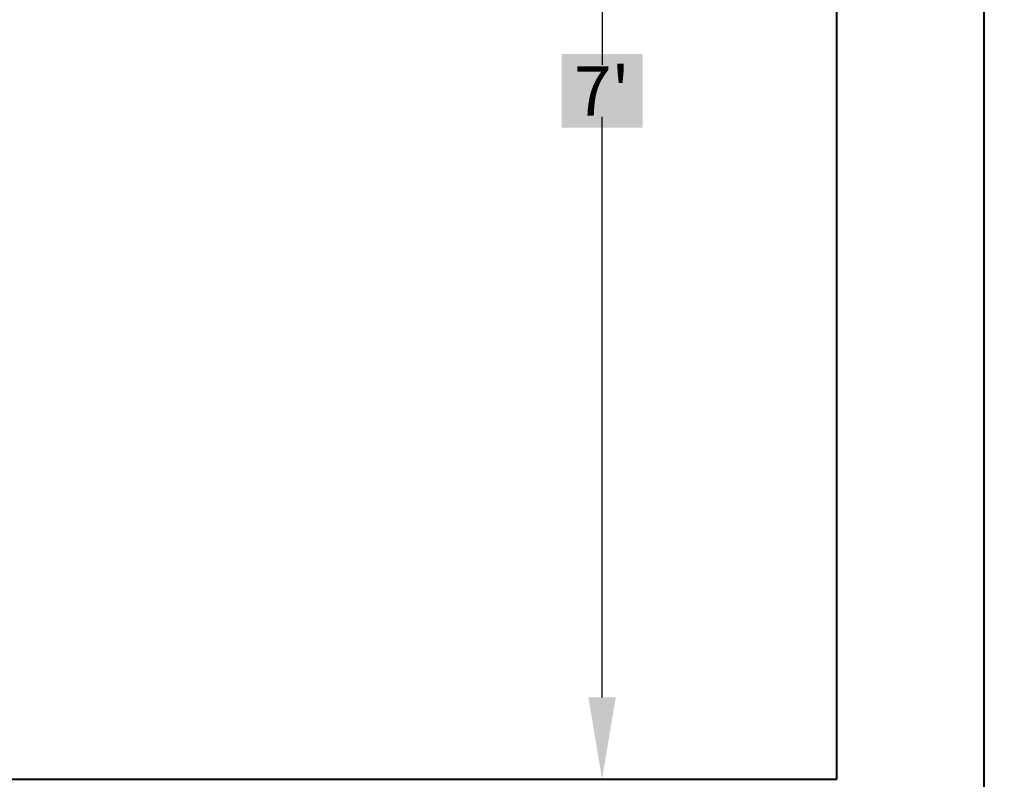
# Model space of a CAD drawing. Units: inches. Extents: x -301 to 715, y -607 to 364.
# Tile 91 of 141: x 74 to 134, y -215 to -168. Entities that reach past the tile are written whole.
import ezdxf

# ---------------------------------------------------------------- set-up
doc = ezdxf.new("R2010")
doc.units = ezdxf.units.IN
doc.header["$MEASUREMENT"] = 0
doc.layers.add('A-ANNO-DIMS', color=2, linetype='Continuous', lineweight=18)
doc.layers.add('A-WALL', color=3, linetype='Continuous', lineweight=40)
doc.styles.get("Standard").update_dxf_attribs({"font": 'arial.ttf'})
doc.dimstyles.get("Standard").update_dxf_attribs({"dimtxt": 0.18, "dimasz": 0.18, "dimexe": 0.18, "dimexo": 0.0625, "dimgap": 0.09, "dimtad": 0, "dimtih": 1, "dimtoh": 1, "dimdec": 1, "dimzin": 0, "dimdsep": 46, "dimlunit": 4, "dimtxsty": 'Standard', "dimcen": 0.09, "dimclrd": 3, "dimclre": 4, "dimclrt": 6, "dimadec": 0, "dimazin": 0, "dimtfac": 1, "dimtdec": 1, "dimtofl": 0, "dimtmove": 0, "dimatfit": 3, "dimfxl": 1, "dimtfill": 2, "dimtfillclr": 51, "dimtolj": 1, "dimtzin": 0, "dimarcsym": 0})

# ---------------------------------------------------------------- blocks, each defined once
blk = doc.blocks.new('*D43')
at = {"layer": 'A-ANNO-DIMS', "color": 0, "lineweight": -2, "transparency": 16777216}
for p, q in [((123.834, -130.818), (109.393, -130.818)), ((109.573, -135.818), (109.573, -171.228)), ((109.573, -209.818), (109.573, -174.408)), ((123.834, -214.818), (109.393, -214.818))]:
    blk.add_line(p, q, dxfattribs=at)
at = {"layer": 'A-ANNO-DIMS', "color": 0, "transparency": 16777216}
for points in [[(108.739, -135.818), (110.406, -135.818), (109.573, -130.818)], [(108.739, -209.818), (110.406, -209.818), (109.573, -214.818)]]:
    blk.add_solid(points, dxfattribs=at)
at = {"layer": 'Defpoints', "color": 0, "transparency": 16777216}
for p in [(123.897, -130.818), (109.573, -214.818), (123.897, -214.818)]:
    blk.add_point(p, dxfattribs=at)
at = {"layer": 'A-ANNO-DIMS', "color": 0, "transparency": 16777216, "insert": (109.573, -172.818), "char_height": 3, "attachment_point": 5, "bg_fill": 1, "box_fill_scale": 1.25, "bg_fill_color": 51, "bg_fill_transparency": 0}
blk.add_mtext("\\A1;7'", dxfattribs=at)
blk = doc.blocks.new('*D152')
at = {"layer": 'A-ANNO-DIMS', "color": 4, "lineweight": -2, "transparency": 16777216}
for p, q in [((123.959, -130.818), (233.659, -130.818)), ((132.959, -223.818), (233.659, -223.818))]:
    blk.add_line(p, q, dxfattribs=at)
at = {"layer": 'A-ANNO-DIMS', "color": 3, "lineweight": -2, "transparency": 16777216}
for p, q in [((233.479, -130.998), (233.479, -177.136)), ((233.479, -223.638), (233.479, -177.5))]:
    blk.add_line(p, q, dxfattribs=at)
at = {"layer": 'A-ANNO-DIMS', "color": 3, "transparency": 16777216}
for points in [[(233.449, -130.998), (233.509, -130.998), (233.479, -130.818)], [(233.449, -223.638), (233.509, -223.638), (233.479, -223.818)]]:
    blk.add_solid(points, dxfattribs=at)
at = {"layer": 'Defpoints', "color": 0, "transparency": 16777216}
for p in [(123.897, -130.818), (233.479, -130.818), (132.897, -223.818)]:
    blk.add_point(p, dxfattribs=at)
at = {"layer": 'A-ANNO-DIMS', "color": 6, "transparency": 16777216, "insert": (233.479, -177.318), "char_height": 0.18, "attachment_point": 5, "bg_fill": 1, "box_fill_scale": 1.25, "bg_fill_color": 51, "bg_fill_transparency": 0}
blk.add_mtext('\\A1;7\'-9"', dxfattribs=at)

msp = doc.modelspace()

# ---------------------------------------------------------------- linework, layer by layer
at = {"layer": 'A-WALL'}
for p, q in [((123.897, -214.818), (123.897, -82.818)), ((132.897, -223.818), (132.897, -124.818)), ((-45.841, -214.818), (123.897, -214.818)), ((123.897, -214.818), (123.897, -214.818))]:
    msp.add_line(p, q, dxfattribs=at)

# ---------------------------------------------------------------- dimensions: what is measured, and where the dimension line sits
at = {"layer": 'A-ANNO-DIMS'}
for base, p1, p2, override, picture, middle in [((109.573, -214.818), (123.897, -130.818), (123.897, -214.818), {"dimtxt": 3, "dimasz": 5, "dimclrd": 0, "dimclre": 0, "dimclrt": 0}, '*D43', (109.573, -172.818)), ((233.479, -130.818), (132.897, -223.818), (123.897, -130.818), {"dimdec": 1, "dimlfac": 1, "dimrnd": 0, "dimzin": 1, "dimdsep": 46, "dimlunit": 4, "dimfrac": 2}, '*D152', (233.479, -177.318))]:
    dim = msp.add_linear_dim(base=base, p1=p1, p2=p2, angle=90, dimstyle='Standard', override=override, dxfattribs=at)
    dim.commit()
    dim.dimension.update_dxf_attribs({"geometry": picture, "text_midpoint": middle})

doc.saveas('drawing.dxf')
